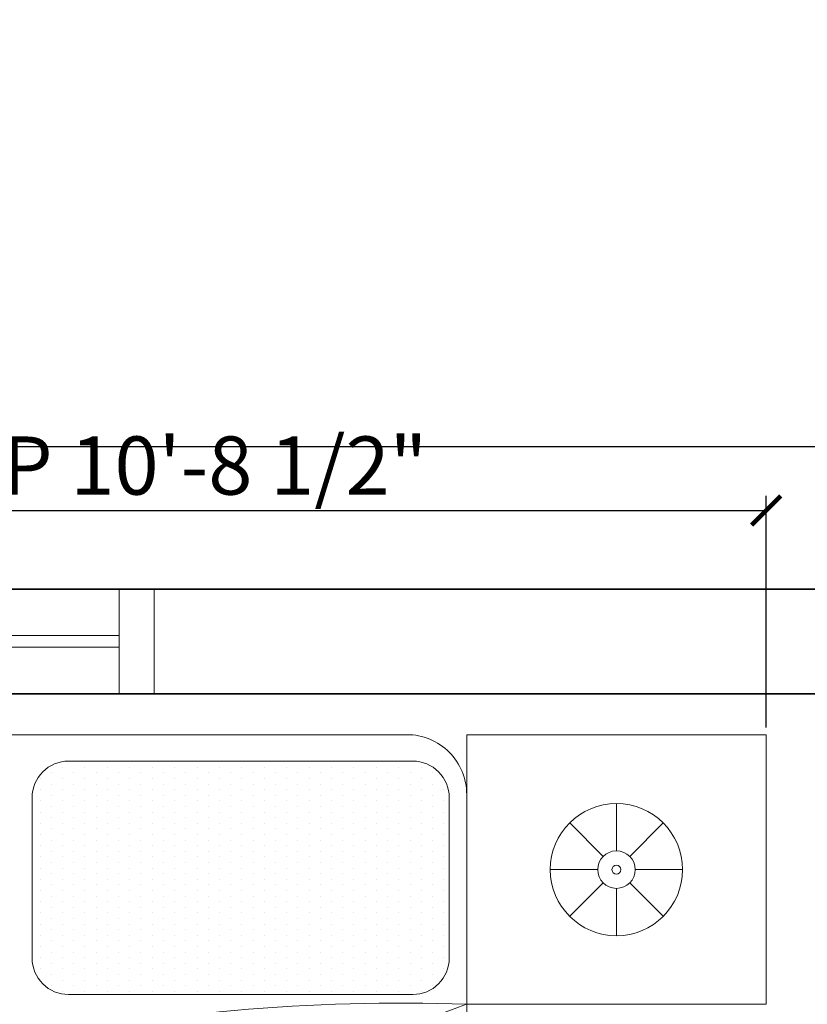
# Model space of a CAD drawing. Units: inches. Extents: x 3283068 to 3284536, y 3240756 to 3241803.
# Tile 11 of 19: x 3283453 to 3283520, y 3241603 to 3241688. Entities that reach past the tile are written whole.
import ezdxf

# ---------------------------------------------------------------- set-up
doc = ezdxf.new("R2010")
doc.units = ezdxf.units.IN
for name, color, linetype, lineweight in [('A-ANNO-DIMS', 2, 'Continuous', 18), ('furniture', 40, 'Continuous', 18), ('wall', 20, 'Continuous', 35), ('window', 100, 'Continuous', 18)]:
    doc.layers.add(name, color=color, linetype=linetype, lineweight=lineweight)
doc.styles.get("Standard").update_dxf_attribs({"font": 'arial.ttf'})
doc.dimstyles.new('ISO-25', dxfattribs={"dimtxt": 5, "dimasz": 2.5, "dimexe": 1.25, "dimexo": 0.625, "dimtad": 1, "dimlunit": 4, "dimtxsty": 'Standard', "dimblk": 'ARCHTICK', "dimcen": 2.5, "dimadec": 0, "dimazin": 0, "dimtfac": 1, "dimtmove": 0, "dimatfit": 3, "dimfxl": 1, "dimarcsym": 0})

# ---------------------------------------------------------------- blocks, each defined once
blk = doc.blocks.new('*X12')
at = {"color": 0}
for p, q in [((273.75, 456.9375), (273.75, 456.9375)), ((273.9375, 457.03125), (273.9375, 457.03125)), ((274.125, 456.9375), (274.125, 456.9375)), ((274.3125, 457.03125), (274.3125, 457.03125)), ((274.5, 456.9375), (274.5, 456.9375)), ((274.6875, 457.03125), (274.6875, 457.03125)), ((274.875, 456.9375), (274.875, 456.9375)), ((275.0625, 457.03125), (275.0625, 457.03125)), ((275.25, 456.9375), (275.25, 456.9375)), ((275.4375, 457.03125), (275.4375, 457.03125)), ((275.625, 456.9375), (275.625, 456.9375)), ((275.8125, 457.03125), (275.8125, 457.03125)), ((276, 456.9375), (276, 456.9375)), ((276.1875, 457.03125), (276.1875, 457.03125)), ((276.375, 456.9375), (276.375, 456.9375)), ((276.5625, 457.03125), (276.5625, 457.03125)), ((276.75, 456.9375), (276.75, 456.9375)), ((276.9375, 457.03125), (276.9375, 457.03125)), ((277.125, 456.9375), (277.125, 456.9375)), ((277.3125, 457.03125), (277.3125, 457.03125)), ((277.5, 456.9375), (277.5, 456.9375)), ((277.6875, 457.03125), (277.6875, 457.03125)), ((277.875, 456.9375), (277.875, 456.9375)), ((278.0625, 457.03125), (278.0625, 457.03125)), ((278.25, 456.9375), (278.25, 456.9375)), ((278.4375, 457.03125), (278.4375, 457.03125)), ((278.625, 456.9375), (278.625, 456.9375)), ((278.8125, 457.03125), (278.8125, 457.03125)), ((279, 456.9375), (279, 456.9375)), ((279.1875, 457.03125), (279.1875, 457.03125)), ((279.375, 456.9375), (279.375, 456.9375)), ((279.5625, 457.03125), (279.5625, 457.03125)), ((279.75, 456.9375), (279.75, 456.9375)), ((273.375, 456.75), (273.375, 456.75)), ((273.5625, 456.84375), (273.5625, 456.84375)), ((273.75, 456.75), (273.75, 456.75)), ((273.9375, 456.84375), (273.9375, 456.84375)), ((274.125, 456.75), (274.125, 456.75)), ((274.3125, 456.84375), (274.3125, 456.84375)), ((274.5, 456.75), (274.5, 456.75)), ((274.6875, 456.84375), (274.6875, 456.84375)), ((274.875, 456.75), (274.875, 456.75)), ((275.0625, 456.84375), (275.0625, 456.84375)), ((275.25, 456.75), (275.25, 456.75)), ((275.4375, 456.84375), (275.4375, 456.84375)), ((275.625, 456.75), (275.625, 456.75)), ((275.8125, 456.84375), (275.8125, 456.84375)), ((276, 456.75), (276, 456.75)), ((276.1875, 456.84375), (276.1875, 456.84375)), ((276.375, 456.75), (276.375, 456.75)), ((276.5625, 456.84375), (276.5625, 456.84375)), ((276.75, 456.75), (276.75, 456.75)), ((276.9375, 456.84375), (276.9375, 456.84375)), ((277.125, 456.75), (277.125, 456.75)), ((277.3125, 456.84375), (277.3125, 456.84375)), ((277.5, 456.75), (277.5, 456.75)), ((277.6875, 456.84375), (277.6875, 456.84375)), ((277.875, 456.75), (277.875, 456.75)), ((278.0625, 456.84375), (278.0625, 456.84375)), ((278.25, 456.75), (278.25, 456.75)), ((278.4375, 456.84375), (278.4375, 456.84375)), ((278.625, 456.75), (278.625, 456.75)), ((278.8125, 456.84375), (278.8125, 456.84375)), ((279, 456.75), (279, 456.75)), ((279.1875, 456.84375), (279.1875, 456.84375)), ((279.375, 456.75), (279.375, 456.75)), ((279.5625, 456.84375), (279.5625, 456.84375)), ((279.75, 456.75), (279.75, 456.75)), ((279.9375, 456.84375), (279.9375, 456.84375)), ((280.125, 456.75), (280.125, 456.75)), ((273.5625, 456.65625), (273.5625, 456.65625)), ((273.9375, 456.65625), (273.9375, 456.65625)), ((274.3125, 456.65625), (274.3125, 456.65625)), ((274.6875, 456.65625), (274.6875, 456.65625)), ((275.0625, 456.65625), (275.0625, 456.65625)), ((275.4375, 456.65625), (275.4375, 456.65625)), ((275.8125, 456.65625), (275.8125, 456.65625)), ((276.1875, 456.65625), (276.1875, 456.65625)), ((276.5625, 456.65625), (276.5625, 456.65625)), ((276.9375, 456.65625), (276.9375, 456.65625)), ((277.3125, 456.65625), (277.3125, 456.65625)), ((277.6875, 456.65625), (277.6875, 456.65625)), ((278.0625, 456.65625), (278.0625, 456.65625)), ((278.4375, 456.65625), (278.4375, 456.65625)), ((278.8125, 456.65625), (278.8125, 456.65625)), ((279.1875, 456.65625), (279.1875, 456.65625)), ((279.5625, 456.65625), (279.5625, 456.65625)), ((279.9375, 456.65625), (279.9375, 456.65625)), ((273.375, 456.5625), (273.375, 456.5625)), ((273.5625, 456.46875), (273.5625, 456.46875)), ((273.75, 456.5625), (273.75, 456.5625)), ((273.9375, 456.46875), (273.9375, 456.46875)), ((274.125, 456.5625), (274.125, 456.5625)), ((274.3125, 456.46875), (274.3125, 456.46875)), ((274.5, 456.5625), (274.5, 456.5625)), ((274.6875, 456.46875), (274.6875, 456.46875)), ((274.875, 456.5625), (274.875, 456.5625)), ((275.0625, 456.46875), (275.0625, 456.46875)), ((275.25, 456.5625), (275.25, 456.5625)), ((275.4375, 456.46875), (275.4375, 456.46875)), ((275.625, 456.5625), (275.625, 456.5625)), ((275.8125, 456.46875), (275.8125, 456.46875)), ((276, 456.5625), (276, 456.5625)), ((276.1875, 456.46875), (276.1875, 456.46875)), ((276.375, 456.5625), (276.375, 456.5625)), ((276.5625, 456.46875), (276.5625, 456.46875)), ((276.75, 456.5625), (276.75, 456.5625)), ((276.9375, 456.46875), (276.9375, 456.46875)), ((277.125, 456.5625), (277.125, 456.5625)), ((277.3125, 456.46875), (277.3125, 456.46875)), ((277.5, 456.5625), (277.5, 456.5625)), ((277.6875, 456.46875), (277.6875, 456.46875)), ((277.875, 456.5625), (277.875, 456.5625)), ((278.0625, 456.46875), (278.0625, 456.46875)), ((278.25, 456.5625), (278.25, 456.5625)), ((278.4375, 456.46875), (278.4375, 456.46875)), ((278.625, 456.5625), (278.625, 456.5625)), ((278.8125, 456.46875), (278.8125, 456.46875)), ((279, 456.5625), (279, 456.5625)), ((279.1875, 456.46875), (279.1875, 456.46875)), ((279.375, 456.5625), (279.375, 456.5625)), ((279.5625, 456.46875), (279.5625, 456.46875)), ((279.75, 456.5625), (279.75, 456.5625)), ((279.9375, 456.46875), (279.9375, 456.46875)), ((280.125, 456.5625), (280.125, 456.5625)), ((273.375, 456.375), (273.375, 456.375)), ((273.5625, 456.28125), (273.5625, 456.28125)), ((273.75, 456.375), (273.75, 456.375)), ((273.9375, 456.28125), (273.9375, 456.28125)), ((274.125, 456.375), (274.125, 456.375)), ((274.3125, 456.28125), (274.3125, 456.28125)), ((274.5, 456.375), (274.5, 456.375)), ((274.6875, 456.28125), (274.6875, 456.28125)), ((274.875, 456.375), (274.875, 456.375)), ((275.0625, 456.28125), (275.0625, 456.28125)), ((275.25, 456.375), (275.25, 456.375)), ((275.4375, 456.28125), (275.4375, 456.28125)), ((275.625, 456.375), (275.625, 456.375)), ((275.8125, 456.28125), (275.8125, 456.28125)), ((276, 456.375), (276, 456.375)), ((276.1875, 456.28125), (276.1875, 456.28125)), ((276.375, 456.375), (276.375, 456.375)), ((276.5625, 456.28125), (276.5625, 456.28125)), ((276.75, 456.375), (276.75, 456.375)), ((276.9375, 456.28125), (276.9375, 456.28125)), ((277.125, 456.375), (277.125, 456.375)), ((277.3125, 456.28125), (277.3125, 456.28125)), ((277.5, 456.375), (277.5, 456.375)), ((277.6875, 456.28125), (277.6875, 456.28125)), ((277.875, 456.375), (277.875, 456.375)), ((278.0625, 456.28125), (278.0625, 456.28125)), ((278.25, 456.375), (278.25, 456.375)), ((278.4375, 456.28125), (278.4375, 456.28125)), ((278.625, 456.375), (278.625, 456.375)), ((278.8125, 456.28125), (278.8125, 456.28125)), ((279, 456.375), (279, 456.375)), ((279.1875, 456.28125), (279.1875, 456.28125)), ((279.375, 456.375), (279.375, 456.375)), ((279.5625, 456.28125), (279.5625, 456.28125)), ((279.75, 456.375), (279.75, 456.375)), ((279.9375, 456.28125), (279.9375, 456.28125)), ((280.125, 456.375), (280.125, 456.375)), ((273.375, 456.1875), (273.375, 456.1875)), ((273.5625, 456.09375), (273.5625, 456.09375)), ((273.75, 456.1875), (273.75, 456.1875)), ((273.9375, 456.09375), (273.9375, 456.09375)), ((274.125, 456.1875), (274.125, 456.1875)), ((274.3125, 456.09375), (274.3125, 456.09375)), ((274.5, 456.1875), (274.5, 456.1875)), ((274.6875, 456.09375), (274.6875, 456.09375)), ((274.875, 456.1875), (274.875, 456.1875)), ((275.0625, 456.09375), (275.0625, 456.09375)), ((275.25, 456.1875), (275.25, 456.1875)), ((275.4375, 456.09375), (275.4375, 456.09375)), ((275.625, 456.1875), (275.625, 456.1875)), ((275.8125, 456.09375), (275.8125, 456.09375)), ((276, 456.1875), (276, 456.1875)), ((276.1875, 456.09375), (276.1875, 456.09375)), ((276.375, 456.1875), (276.375, 456.1875)), ((276.5625, 456.09375), (276.5625, 456.09375)), ((276.75, 456.1875), (276.75, 456.1875)), ((276.9375, 456.09375), (276.9375, 456.09375)), ((277.125, 456.1875), (277.125, 456.1875)), ((277.3125, 456.09375), (277.3125, 456.09375)), ((277.5, 456.1875), (277.5, 456.1875)), ((277.6875, 456.09375), (277.6875, 456.09375)), ((277.875, 456.1875), (277.875, 456.1875)), ((278.0625, 456.09375), (278.0625, 456.09375)), ((278.25, 456.1875), (278.25, 456.1875)), ((278.4375, 456.09375), (278.4375, 456.09375)), ((278.625, 456.1875), (278.625, 456.1875)), ((278.8125, 456.09375), (278.8125, 456.09375)), ((279, 456.1875), (279, 456.1875)), ((279.1875, 456.09375), (279.1875, 456.09375)), ((279.375, 456.1875), (279.375, 456.1875)), ((279.5625, 456.09375), (279.5625, 456.09375)), ((279.75, 456.1875), (279.75, 456.1875)), ((279.9375, 456.09375), (279.9375, 456.09375)), ((280.125, 456.1875), (280.125, 456.1875)), ((273.375, 456), (273.375, 456)), ((273.75, 456), (273.75, 456)), ((274.125, 456), (274.125, 456)), ((274.5, 456), (274.5, 456)), ((274.875, 456), (274.875, 456)), ((275.25, 456), (275.25, 456)), ((275.625, 456), (275.625, 456)), ((276, 456), (276, 456)), ((276.375, 456), (276.375, 456)), ((276.75, 456), (276.75, 456)), ((277.125, 456), (277.125, 456)), ((277.5, 456), (277.5, 456)), ((277.875, 456), (277.875, 456)), ((278.25, 456), (278.25, 456)), ((278.625, 456), (278.625, 456)), ((279, 456), (279, 456)), ((279.375, 456), (279.375, 456)), ((279.75, 456), (279.75, 456)), ((280.125, 456), (280.125, 456)), ((273.375, 455.8125), (273.375, 455.8125)), ((273.5625, 455.90625), (273.5625, 455.90625)), ((273.75, 455.8125), (273.75, 455.8125)), ((273.9375, 455.90625), (273.9375, 455.90625)), ((274.125, 455.8125), (274.125, 455.8125)), ((274.3125, 455.90625), (274.3125, 455.90625)), ((274.5, 455.8125), (274.5, 455.8125)), ((274.6875, 455.90625), (274.6875, 455.90625)), ((274.875, 455.8125), (274.875, 455.8125)), ((275.0625, 455.90625), (275.0625, 455.90625)), ((275.25, 455.8125), (275.25, 455.8125)), ((275.4375, 455.90625), (275.4375, 455.90625)), ((275.625, 455.8125), (275.625, 455.8125)), ((275.8125, 455.90625), (275.8125, 455.90625)), ((276, 455.8125), (276, 455.8125)), ((276.1875, 455.90625), (276.1875, 455.90625)), ((276.375, 455.8125), (276.375, 455.8125)), ((276.5625, 455.90625), (276.5625, 455.90625)), ((276.75, 455.8125), (276.75, 455.8125)), ((276.9375, 455.90625), (276.9375, 455.90625)), ((277.125, 455.8125), (277.125, 455.8125)), ((277.3125, 455.90625), (277.3125, 455.90625)), ((277.5, 455.8125), (277.5, 455.8125)), ((277.6875, 455.90625), (277.6875, 455.90625)), ((277.875, 455.8125), (277.875, 455.8125)), ((278.0625, 455.90625), (278.0625, 455.90625)), ((278.25, 455.8125), (278.25, 455.8125)), ((278.4375, 455.90625), (278.4375, 455.90625)), ((278.625, 455.8125), (278.625, 455.8125)), ((278.8125, 455.90625), (278.8125, 455.90625)), ((279, 455.8125), (279, 455.8125)), ((279.1875, 455.90625), (279.1875, 455.90625)), ((279.375, 455.8125), (279.375, 455.8125)), ((279.5625, 455.90625), (279.5625, 455.90625)), ((279.75, 455.8125), (279.75, 455.8125)), ((279.9375, 455.90625), (279.9375, 455.90625)), ((280.125, 455.8125), (280.125, 455.8125)), ((273.375, 455.625), (273.375, 455.625)), ((273.5625, 455.71875), (273.5625, 455.71875)), ((273.75, 455.625), (273.75, 455.625)), ((273.9375, 455.71875), (273.9375, 455.71875)), ((274.125, 455.625), (274.125, 455.625)), ((274.3125, 455.71875), (274.3125, 455.71875)), ((274.5, 455.625), (274.5, 455.625)), ((274.6875, 455.71875), (274.6875, 455.71875)), ((274.875, 455.625), (274.875, 455.625)), ((275.0625, 455.71875), (275.0625, 455.71875)), ((275.25, 455.625), (275.25, 455.625)), ((275.4375, 455.71875), (275.4375, 455.71875)), ((275.625, 455.625), (275.625, 455.625)), ((275.8125, 455.71875), (275.8125, 455.71875)), ((276, 455.625), (276, 455.625)), ((276.1875, 455.71875), (276.1875, 455.71875)), ((276.375, 455.625), (276.375, 455.625)), ((276.5625, 455.71875), (276.5625, 455.71875)), ((276.75, 455.625), (276.75, 455.625)), ((276.9375, 455.71875), (276.9375, 455.71875)), ((277.125, 455.625), (277.125, 455.625)), ((277.3125, 455.71875), (277.3125, 455.71875)), ((277.5, 455.625), (277.5, 455.625)), ((277.6875, 455.71875), (277.6875, 455.71875)), ((277.875, 455.625), (277.875, 455.625)), ((278.0625, 455.71875), (278.0625, 455.71875)), ((278.25, 455.625), (278.25, 455.625)), ((278.4375, 455.71875), (278.4375, 455.71875)), ((278.625, 455.625), (278.625, 455.625)), ((278.8125, 455.71875), (278.8125, 455.71875)), ((279, 455.625), (279, 455.625)), ((279.1875, 455.71875), (279.1875, 455.71875)), ((279.375, 455.625), (279.375, 455.625)), ((279.5625, 455.71875), (279.5625, 455.71875)), ((279.75, 455.625), (279.75, 455.625)), ((279.9375, 455.71875), (279.9375, 455.71875)), ((280.125, 455.625), (280.125, 455.625)), ((273.375, 455.4375), (273.375, 455.4375)), ((273.5625, 455.53125), (273.5625, 455.53125)), ((273.75, 455.4375), (273.75, 455.4375)), ((273.9375, 455.53125), (273.9375, 455.53125)), ((274.125, 455.4375), (274.125, 455.4375)), ((274.3125, 455.53125), (274.3125, 455.53125)), ((274.5, 455.4375), (274.5, 455.4375)), ((274.6875, 455.53125), (274.6875, 455.53125)), ((274.875, 455.4375), (274.875, 455.4375)), ((275.0625, 455.53125), (275.0625, 455.53125)), ((275.25, 455.4375), (275.25, 455.4375)), ((275.4375, 455.53125), (275.4375, 455.53125)), ((275.625, 455.4375), (275.625, 455.4375)), ((275.8125, 455.53125), (275.8125, 455.53125)), ((276, 455.4375), (276, 455.4375)), ((276.1875, 455.53125), (276.1875, 455.53125)), ((276.375, 455.4375), (276.375, 455.4375)), ((276.5625, 455.53125), (276.5625, 455.53125)), ((276.75, 455.4375), (276.75, 455.4375)), ((276.9375, 455.53125), (276.9375, 455.53125)), ((277.125, 455.4375), (277.125, 455.4375)), ((277.3125, 455.53125), (277.3125, 455.53125)), ((277.5, 455.4375), (277.5, 455.4375)), ((277.6875, 455.53125), (277.6875, 455.53125)), ((277.875, 455.4375), (277.875, 455.4375)), ((278.0625, 455.53125), (278.0625, 455.53125)), ((278.25, 455.4375), (278.25, 455.4375)), ((278.4375, 455.53125), (278.4375, 455.53125)), ((278.625, 455.4375), (278.625, 455.4375)), ((278.8125, 455.53125), (278.8125, 455.53125)), ((279, 455.4375), (279, 455.4375)), ((279.1875, 455.53125), (279.1875, 455.53125)), ((279.375, 455.4375), (279.375, 455.4375)), ((279.5625, 455.53125), (279.5625, 455.53125)), ((279.75, 455.4375), (279.75, 455.4375)), ((279.9375, 455.53125), (279.9375, 455.53125)), ((280.125, 455.4375), (280.125, 455.4375)), ((273.5625, 455.34375), (273.5625, 455.34375)), ((273.9375, 455.34375), (273.9375, 455.34375)), ((274.3125, 455.34375), (274.3125, 455.34375)), ((274.6875, 455.34375), (274.6875, 455.34375)), ((275.0625, 455.34375), (275.0625, 455.34375)), ((275.4375, 455.34375), (275.4375, 455.34375)), ((275.8125, 455.34375), (275.8125, 455.34375)), ((276.1875, 455.34375), (276.1875, 455.34375)), ((276.5625, 455.34375), (276.5625, 455.34375)), ((276.9375, 455.34375), (276.9375, 455.34375)), ((277.3125, 455.34375), (277.3125, 455.34375)), ((277.6875, 455.34375), (277.6875, 455.34375)), ((278.0625, 455.34375), (278.0625, 455.34375)), ((278.4375, 455.34375), (278.4375, 455.34375)), ((278.8125, 455.34375), (278.8125, 455.34375)), ((279.1875, 455.34375), (279.1875, 455.34375)), ((279.5625, 455.34375), (279.5625, 455.34375)), ((279.9375, 455.34375), (279.9375, 455.34375)), ((273.375, 455.25), (273.375, 455.25)), ((273.5625, 455.15625), (273.5625, 455.15625)), ((273.75, 455.25), (273.75, 455.25)), ((273.9375, 455.15625), (273.9375, 455.15625)), ((274.125, 455.25), (274.125, 455.25)), ((274.3125, 455.15625), (274.3125, 455.15625)), ((274.5, 455.25), (274.5, 455.25)), ((274.6875, 455.15625), (274.6875, 455.15625)), ((274.875, 455.25), (274.875, 455.25)), ((275.0625, 455.15625), (275.0625, 455.15625)), ((275.25, 455.25), (275.25, 455.25)), ((275.4375, 455.15625), (275.4375, 455.15625)), ((275.625, 455.25), (275.625, 455.25)), ((275.8125, 455.15625), (275.8125, 455.15625)), ((276, 455.25), (276, 455.25)), ((276.1875, 455.15625), (276.1875, 455.15625)), ((276.375, 455.25), (276.375, 455.25)), ((276.5625, 455.15625), (276.5625, 455.15625)), ((276.75, 455.25), (276.75, 455.25)), ((276.9375, 455.15625), (276.9375, 455.15625)), ((277.125, 455.25), (277.125, 455.25)), ((277.3125, 455.15625), (277.3125, 455.15625)), ((277.5, 455.25), (277.5, 455.25)), ((277.6875, 455.15625), (277.6875, 455.15625)), ((277.875, 455.25), (277.875, 455.25)), ((278.0625, 455.15625), (278.0625, 455.15625)), ((278.25, 455.25), (278.25, 455.25)), ((278.4375, 455.15625), (278.4375, 455.15625)), ((278.625, 455.25), (278.625, 455.25)), ((278.8125, 455.15625), (278.8125, 455.15625)), ((279, 455.25), (279, 455.25)), ((279.1875, 455.15625), (279.1875, 455.15625)), ((279.375, 455.25), (279.375, 455.25)), ((279.5625, 455.15625), (279.5625, 455.15625)), ((279.75, 455.25), (279.75, 455.25)), ((279.9375, 455.15625), (279.9375, 455.15625)), ((280.125, 455.25), (280.125, 455.25)), ((273.375, 455.0625), (273.375, 455.0625)), ((273.5625, 454.96875), (273.5625, 454.96875)), ((273.75, 455.0625), (273.75, 455.0625)), ((273.9375, 454.96875), (273.9375, 454.96875)), ((274.125, 455.0625), (274.125, 455.0625)), ((274.3125, 454.96875), (274.3125, 454.96875)), ((274.5, 455.0625), (274.5, 455.0625)), ((274.6875, 454.96875), (274.6875, 454.96875)), ((274.875, 455.0625), (274.875, 455.0625)), ((275.0625, 454.96875), (275.0625, 454.96875)), ((275.25, 455.0625), (275.25, 455.0625)), ((275.4375, 454.96875), (275.4375, 454.96875)), ((275.625, 455.0625), (275.625, 455.0625)), ((275.8125, 454.96875), (275.8125, 454.96875)), ((276, 455.0625), (276, 455.0625)), ((276.1875, 454.96875), (276.1875, 454.96875)), ((276.375, 455.0625), (276.375, 455.0625)), ((276.5625, 454.96875), (276.5625, 454.96875)), ((276.75, 455.0625), (276.75, 455.0625)), ((276.9375, 454.96875), (276.9375, 454.96875)), ((277.125, 455.0625), (277.125, 455.0625)), ((277.3125, 454.96875), (277.3125, 454.96875)), ((277.5, 455.0625), (277.5, 455.0625)), ((277.6875, 454.96875), (277.6875, 454.96875)), ((277.875, 455.0625), (277.875, 455.0625)), ((278.0625, 454.96875), (278.0625, 454.96875)), ((278.25, 455.0625), (278.25, 455.0625)), ((278.4375, 454.96875), (278.4375, 454.96875)), ((278.625, 455.0625), (278.625, 455.0625)), ((278.8125, 454.96875), (278.8125, 454.96875)), ((279, 455.0625), (279, 455.0625)), ((279.1875, 454.96875), (279.1875, 454.96875)), ((279.375, 455.0625), (279.375, 455.0625)), ((279.5625, 454.96875), (279.5625, 454.96875)), ((279.75, 455.0625), (279.75, 455.0625)), ((279.9375, 454.96875), (279.9375, 454.96875)), ((280.125, 455.0625), (280.125, 455.0625)), ((273.375, 454.875), (273.375, 454.875)), ((273.5625, 454.78125), (273.5625, 454.78125)), ((273.75, 454.875), (273.75, 454.875)), ((273.9375, 454.78125), (273.9375, 454.78125)), ((274.125, 454.875), (274.125, 454.875)), ((274.3125, 454.78125), (274.3125, 454.78125)), ((274.5, 454.875), (274.5, 454.875)), ((274.6875, 454.78125), (274.6875, 454.78125)), ((274.875, 454.875), (274.875, 454.875)), ((275.0625, 454.78125), (275.0625, 454.78125)), ((275.25, 454.875), (275.25, 454.875)), ((275.4375, 454.78125), (275.4375, 454.78125)), ((275.625, 454.875), (275.625, 454.875)), ((275.8125, 454.78125), (275.8125, 454.78125)), ((276, 454.875), (276, 454.875)), ((276.1875, 454.78125), (276.1875, 454.78125)), ((276.375, 454.875), (276.375, 454.875)), ((276.5625, 454.78125), (276.5625, 454.78125)), ((276.75, 454.875), (276.75, 454.875)), ((276.9375, 454.78125), (276.9375, 454.78125)), ((277.125, 454.875), (277.125, 454.875)), ((277.3125, 454.78125), (277.3125, 454.78125)), ((277.5, 454.875), (277.5, 454.875)), ((277.6875, 454.78125), (277.6875, 454.78125)), ((277.875, 454.875), (277.875, 454.875)), ((278.0625, 454.78125), (278.0625, 454.78125)), ((278.25, 454.875), (278.25, 454.875)), ((278.4375, 454.78125), (278.4375, 454.78125)), ((278.625, 454.875), (278.625, 454.875)), ((278.8125, 454.78125), (278.8125, 454.78125)), ((279, 454.875), (279, 454.875)), ((279.1875, 454.78125), (279.1875, 454.78125)), ((279.375, 454.875), (279.375, 454.875)), ((279.5625, 454.78125), (279.5625, 454.78125)), ((279.75, 454.875), (279.75, 454.875)), ((279.9375, 454.78125), (279.9375, 454.78125)), ((280.125, 454.875), (280.125, 454.875)), ((273.375, 454.6875), (273.375, 454.6875)), ((273.75, 454.6875), (273.75, 454.6875)), ((274.125, 454.6875), (274.125, 454.6875)), ((274.5, 454.6875), (274.5, 454.6875)), ((274.875, 454.6875), (274.875, 454.6875)), ((275.25, 454.6875), (275.25, 454.6875)), ((275.625, 454.6875), (275.625, 454.6875)), ((276, 454.6875), (276, 454.6875)), ((276.375, 454.6875), (276.375, 454.6875)), ((276.75, 454.6875), (276.75, 454.6875)), ((277.125, 454.6875), (277.125, 454.6875)), ((277.5, 454.6875), (277.5, 454.6875)), ((277.875, 454.6875), (277.875, 454.6875)), ((278.25, 454.6875), (278.25, 454.6875)), ((278.625, 454.6875), (278.625, 454.6875)), ((279, 454.6875), (279, 454.6875)), ((279.375, 454.6875), (279.375, 454.6875)), ((279.75, 454.6875), (279.75, 454.6875)), ((280.125, 454.6875), (280.125, 454.6875)), ((273.375, 454.5), (273.375, 454.5)), ((273.5625, 454.59375), (273.5625, 454.59375)), ((273.75, 454.5), (273.75, 454.5)), ((273.9375, 454.59375), (273.9375, 454.59375)), ((274.125, 454.5), (274.125, 454.5)), ((274.3125, 454.59375), (274.3125, 454.59375)), ((274.5, 454.5), (274.5, 454.5)), ((274.6875, 454.59375), (274.6875, 454.59375)), ((274.875, 454.5), (274.875, 454.5)), ((275.0625, 454.59375), (275.0625, 454.59375)), ((275.25, 454.5), (275.25, 454.5)), ((275.4375, 454.59375), (275.4375, 454.59375)), ((275.625, 454.5), (275.625, 454.5)), ((275.8125, 454.59375), (275.8125, 454.59375)), ((276, 454.5), (276, 454.5)), ((276.1875, 454.59375), (276.1875, 454.59375)), ((276.375, 454.5), (276.375, 454.5)), ((276.5625, 454.59375), (276.5625, 454.59375)), ((276.75, 454.5), (276.75, 454.5)), ((276.9375, 454.59375), (276.9375, 454.59375)), ((277.125, 454.5), (277.125, 454.5)), ((277.3125, 454.59375), (277.3125, 454.59375)), ((277.5, 454.5), (277.5, 454.5)), ((277.6875, 454.59375), (277.6875, 454.59375)), ((277.875, 454.5), (277.875, 454.5)), ((278.0625, 454.59375), (278.0625, 454.59375)), ((278.25, 454.5), (278.25, 454.5)), ((278.4375, 454.59375), (278.4375, 454.59375)), ((278.625, 454.5), (278.625, 454.5)), ((278.8125, 454.59375), (278.8125, 454.59375)), ((279, 454.5), (279, 454.5)), ((279.1875, 454.59375), (279.1875, 454.59375)), ((279.375, 454.5), (279.375, 454.5)), ((279.5625, 454.59375), (279.5625, 454.59375)), ((279.75, 454.5), (279.75, 454.5)), ((279.9375, 454.59375), (279.9375, 454.59375)), ((280.125, 454.5), (280.125, 454.5)), ((273.375, 454.3125), (273.375, 454.3125)), ((273.5625, 454.40625), (273.5625, 454.40625)), ((273.75, 454.3125), (273.75, 454.3125)), ((273.9375, 454.40625), (273.9375, 454.40625)), ((274.125, 454.3125), (274.125, 454.3125)), ((274.3125, 454.40625), (274.3125, 454.40625)), ((274.5, 454.3125), (274.5, 454.3125)), ((274.6875, 454.40625), (274.6875, 454.40625)), ((274.875, 454.3125), (274.875, 454.3125)), ((275.0625, 454.40625), (275.0625, 454.40625)), ((275.25, 454.3125), (275.25, 454.3125)), ((275.4375, 454.40625), (275.4375, 454.40625)), ((275.625, 454.3125), (275.625, 454.3125)), ((275.8125, 454.40625), (275.8125, 454.40625)), ((276, 454.3125), (276, 454.3125)), ((276.1875, 454.40625), (276.1875, 454.40625)), ((276.375, 454.3125), (276.375, 454.3125)), ((276.5625, 454.40625), (276.5625, 454.40625)), ((276.75, 454.3125), (276.75, 454.3125)), ((276.9375, 454.40625), (276.9375, 454.40625)), ((277.125, 454.3125), (277.125, 454.3125)), ((277.3125, 454.40625), (277.3125, 454.40625)), ((277.5, 454.3125), (277.5, 454.3125)), ((277.6875, 454.40625), (277.6875, 454.40625)), ((277.875, 454.3125), (277.875, 454.3125)), ((278.0625, 454.40625), (278.0625, 454.40625)), ((278.25, 454.3125), (278.25, 454.3125)), ((278.4375, 454.40625), (278.4375, 454.40625)), ((278.625, 454.3125), (278.625, 454.3125)), ((278.8125, 454.40625), (278.8125, 454.40625)), ((279, 454.3125), (279, 454.3125)), ((279.1875, 454.40625), (279.1875, 454.40625)), ((279.375, 454.3125), (279.375, 454.3125)), ((279.5625, 454.40625), (279.5625, 454.40625)), ((279.75, 454.3125), (279.75, 454.3125)), ((279.9375, 454.40625), (279.9375, 454.40625)), ((280.125, 454.3125), (280.125, 454.3125)), ((273.375, 454.125), (273.375, 454.125)), ((273.5625, 454.21875), (273.5625, 454.21875)), ((273.75, 454.125), (273.75, 454.125)), ((273.9375, 454.21875), (273.9375, 454.21875)), ((274.125, 454.125), (274.125, 454.125)), ((274.3125, 454.21875), (274.3125, 454.21875)), ((274.5, 454.125), (274.5, 454.125)), ((274.6875, 454.21875), (274.6875, 454.21875)), ((274.875, 454.125), (274.875, 454.125)), ((275.0625, 454.21875), (275.0625, 454.21875)), ((275.25, 454.125), (275.25, 454.125)), ((275.4375, 454.21875), (275.4375, 454.21875)), ((275.625, 454.125), (275.625, 454.125)), ((275.8125, 454.21875), (275.8125, 454.21875)), ((276, 454.125), (276, 454.125)), ((276.1875, 454.21875), (276.1875, 454.21875)), ((276.375, 454.125), (276.375, 454.125)), ((276.5625, 454.21875), (276.5625, 454.21875)), ((276.75, 454.125), (276.75, 454.125)), ((276.9375, 454.21875), (276.9375, 454.21875)), ((277.125, 454.125), (277.125, 454.125)), ((277.3125, 454.21875), (277.3125, 454.21875)), ((277.5, 454.125), (277.5, 454.125)), ((277.6875, 454.21875), (277.6875, 454.21875)), ((277.875, 454.125), (277.875, 454.125)), ((278.0625, 454.21875), (278.0625, 454.21875)), ((278.25, 454.125), (278.25, 454.125)), ((278.4375, 454.21875), (278.4375, 454.21875)), ((278.625, 454.125), (278.625, 454.125)), ((278.8125, 454.21875), (278.8125, 454.21875)), ((279, 454.125), (279, 454.125)), ((279.1875, 454.21875), (279.1875, 454.21875)), ((279.375, 454.125), (279.375, 454.125)), ((279.5625, 454.21875), (279.5625, 454.21875)), ((279.75, 454.125), (279.75, 454.125)), ((279.9375, 454.21875), (279.9375, 454.21875)), ((280.125, 454.125), (280.125, 454.125)), ((273.5625, 454.03125), (273.5625, 454.03125)), ((273.9375, 454.03125), (273.9375, 454.03125)), ((274.3125, 454.03125), (274.3125, 454.03125)), ((274.6875, 454.03125), (274.6875, 454.03125)), ((275.0625, 454.03125), (275.0625, 454.03125)), ((275.4375, 454.03125), (275.4375, 454.03125)), ((275.8125, 454.03125), (275.8125, 454.03125)), ((276.1875, 454.03125), (276.1875, 454.03125)), ((276.5625, 454.03125), (276.5625, 454.03125)), ((276.9375, 454.03125), (276.9375, 454.03125)), ((277.3125, 454.03125), (277.3125, 454.03125)), ((277.6875, 454.03125), (277.6875, 454.03125)), ((278.0625, 454.03125), (278.0625, 454.03125)), ((278.4375, 454.03125), (278.4375, 454.03125)), ((278.8125, 454.03125), (278.8125, 454.03125)), ((279.1875, 454.03125), (279.1875, 454.03125)), ((279.5625, 454.03125), (279.5625, 454.03125)), ((279.9375, 454.03125), (279.9375, 454.03125)), ((273.375, 453.9375), (273.375, 453.9375)), ((273.5625, 453.84375), (273.5625, 453.84375)), ((273.75, 453.9375), (273.75, 453.9375)), ((273.9375, 453.84375), (273.9375, 453.84375)), ((274.125, 453.9375), (274.125, 453.9375)), ((274.3125, 453.84375), (274.3125, 453.84375)), ((274.5, 453.9375), (274.5, 453.9375)), ((274.6875, 453.84375), (274.6875, 453.84375)), ((274.875, 453.9375), (274.875, 453.9375)), ((275.0625, 453.84375), (275.0625, 453.84375)), ((275.25, 453.9375), (275.25, 453.9375)), ((275.4375, 453.84375), (275.4375, 453.84375)), ((275.625, 453.9375), (275.625, 453.9375)), ((275.8125, 453.84375), (275.8125, 453.84375)), ((276, 453.9375), (276, 453.9375)), ((276.1875, 453.84375), (276.1875, 453.84375)), ((276.375, 453.9375), (276.375, 453.9375)), ((276.5625, 453.84375), (276.5625, 453.84375)), ((276.75, 453.9375), (276.75, 453.9375)), ((276.9375, 453.84375), (276.9375, 453.84375)), ((277.125, 453.9375), (277.125, 453.9375)), ((277.3125, 453.84375), (277.3125, 453.84375)), ((277.5, 453.9375), (277.5, 453.9375)), ((277.6875, 453.84375), (277.6875, 453.84375)), ((277.875, 453.9375), (277.875, 453.9375)), ((278.0625, 453.84375), (278.0625, 453.84375)), ((278.25, 453.9375), (278.25, 453.9375)), ((278.4375, 453.84375), (278.4375, 453.84375)), ((278.625, 453.9375), (278.625, 453.9375)), ((278.8125, 453.84375), (278.8125, 453.84375)), ((279, 453.9375), (279, 453.9375)), ((279.1875, 453.84375), (279.1875, 453.84375)), ((279.375, 453.9375), (279.375, 453.9375)), ((279.5625, 453.84375), (279.5625, 453.84375)), ((279.75, 453.9375), (279.75, 453.9375)), ((279.9375, 453.84375), (279.9375, 453.84375)), ((280.125, 453.9375), (280.125, 453.9375)), ((273.375, 453.75), (273.375, 453.75)), ((273.5625, 453.65625), (273.5625, 453.65625)), ((273.75, 453.75), (273.75, 453.75)), ((273.9375, 453.65625), (273.9375, 453.65625)), ((274.125, 453.75), (274.125, 453.75)), ((274.3125, 453.65625), (274.3125, 453.65625)), ((274.5, 453.75), (274.5, 453.75)), ((274.6875, 453.65625), (274.6875, 453.65625)), ((274.875, 453.75), (274.875, 453.75)), ((275.0625, 453.65625), (275.0625, 453.65625)), ((275.25, 453.75), (275.25, 453.75)), ((275.4375, 453.65625), (275.4375, 453.65625)), ((275.625, 453.75), (275.625, 453.75)), ((275.8125, 453.65625), (275.8125, 453.65625)), ((276, 453.75), (276, 453.75)), ((276.1875, 453.65625), (276.1875, 453.65625)), ((276.375, 453.75), (276.375, 453.75)), ((276.5625, 453.65625), (276.5625, 453.65625)), ((276.75, 453.75), (276.75, 453.75)), ((276.9375, 453.65625), (276.9375, 453.65625)), ((277.125, 453.75), (277.125, 453.75)), ((277.3125, 453.65625), (277.3125, 453.65625)), ((277.5, 453.75), (277.5, 453.75)), ((277.6875, 453.65625), (277.6875, 453.65625)), ((277.875, 453.75), (277.875, 453.75)), ((278.0625, 453.65625), (278.0625, 453.65625)), ((278.25, 453.75), (278.25, 453.75)), ((278.4375, 453.65625), (278.4375, 453.65625)), ((278.625, 453.75), (278.625, 453.75)), ((278.8125, 453.65625), (278.8125, 453.65625)), ((279, 453.75), (279, 453.75)), ((279.1875, 453.65625), (279.1875, 453.65625)), ((279.375, 453.75), (279.375, 453.75)), ((279.5625, 453.65625), (279.5625, 453.65625)), ((279.75, 453.75), (279.75, 453.75)), ((279.9375, 453.65625), (279.9375, 453.65625)), ((280.125, 453.75), (280.125, 453.75)), ((273.375, 453.5625), (273.375, 453.5625)), ((273.5625, 453.46875), (273.5625, 453.46875)), ((273.75, 453.5625), (273.75, 453.5625)), ((273.9375, 453.46875), (273.9375, 453.46875)), ((274.125, 453.5625), (274.125, 453.5625)), ((274.3125, 453.46875), (274.3125, 453.46875)), ((274.5, 453.5625), (274.5, 453.5625)), ((274.6875, 453.46875), (274.6875, 453.46875)), ((274.875, 453.5625), (274.875, 453.5625)), ((275.0625, 453.46875), (275.0625, 453.46875)), ((275.25, 453.5625), (275.25, 453.5625)), ((275.4375, 453.46875), (275.4375, 453.46875)), ((275.625, 453.5625), (275.625, 453.5625)), ((275.8125, 453.46875), (275.8125, 453.46875)), ((276, 453.5625), (276, 453.5625)), ((276.1875, 453.46875), (276.1875, 453.46875)), ((276.375, 453.5625), (276.375, 453.5625)), ((276.5625, 453.46875), (276.5625, 453.46875)), ((276.75, 453.5625), (276.75, 453.5625)), ((276.9375, 453.46875), (276.9375, 453.46875)), ((277.125, 453.5625), (277.125, 453.5625)), ((277.3125, 453.46875), (277.3125, 453.46875)), ((277.5, 453.5625), (277.5, 453.5625)), ((277.6875, 453.46875), (277.6875, 453.46875)), ((277.875, 453.5625), (277.875, 453.5625)), ((278.0625, 453.46875), (278.0625, 453.46875)), ((278.25, 453.5625), (278.25, 453.5625)), ((278.4375, 453.46875), (278.4375, 453.46875)), ((278.625, 453.5625), (278.625, 453.5625)), ((278.8125, 453.46875), (278.8125, 453.46875)), ((279, 453.5625), (279, 453.5625)), ((279.1875, 453.46875), (279.1875, 453.46875)), ((279.375, 453.5625), (279.375, 453.5625)), ((279.5625, 453.46875), (279.5625, 453.46875)), ((279.75, 453.5625), (279.75, 453.5625)), ((279.9375, 453.46875), (279.9375, 453.46875)), ((280.125, 453.5625), (280.125, 453.5625)), ((273.375, 453.375), (273.375, 453.375)), ((273.75, 453.375), (273.75, 453.375)), ((274.125, 453.375), (274.125, 453.375)), ((274.5, 453.375), (274.5, 453.375)), ((274.875, 453.375), (274.875, 453.375)), ((275.25, 453.375), (275.25, 453.375)), ((275.625, 453.375), (275.625, 453.375)), ((276, 453.375), (276, 453.375)), ((276.375, 453.375), (276.375, 453.375)), ((276.75, 453.375), (276.75, 453.375)), ((277.125, 453.375), (277.125, 453.375)), ((277.5, 453.375), (277.5, 453.375)), ((277.875, 453.375), (277.875, 453.375)), ((278.25, 453.375), (278.25, 453.375)), ((278.625, 453.375), (278.625, 453.375)), ((279, 453.375), (279, 453.375)), ((279.375, 453.375), (279.375, 453.375)), ((279.75, 453.375), (279.75, 453.375)), ((273.5625, 453.28125), (273.5625, 453.28125)), ((273.75, 453.1875), (273.75, 453.1875)), ((273.9375, 453.28125), (273.9375, 453.28125)), ((274.125, 453.1875), (274.125, 453.1875)), ((274.3125, 453.28125), (274.3125, 453.28125)), ((274.5, 453.1875), (274.5, 453.1875)), ((274.6875, 453.28125), (274.6875, 453.28125)), ((274.875, 453.1875), (274.875, 453.1875)), ((275.0625, 453.28125), (275.0625, 453.28125)), ((275.25, 453.1875), (275.25, 453.1875)), ((275.4375, 453.28125), (275.4375, 453.28125)), ((275.625, 453.1875), (275.625, 453.1875)), ((275.8125, 453.28125), (275.8125, 453.28125)), ((276, 453.1875), (276, 453.1875)), ((276.1875, 453.28125), (276.1875, 453.28125)), ((276.375, 453.1875), (276.375, 453.1875)), ((276.5625, 453.28125), (276.5625, 453.28125)), ((276.75, 453.1875), (276.75, 453.1875)), ((276.9375, 453.28125), (276.9375, 453.28125)), ((277.125, 453.1875), (277.125, 453.1875)), ((277.3125, 453.28125), (277.3125, 453.28125)), ((277.5, 453.1875), (277.5, 453.1875)), ((277.6875, 453.28125), (277.6875, 453.28125)), ((277.875, 453.1875), (277.875, 453.1875)), ((278.0625, 453.28125), (278.0625, 453.28125)), ((278.25, 453.1875), (278.25, 453.1875)), ((278.4375, 453.28125), (278.4375, 453.28125)), ((278.625, 453.1875), (278.625, 453.1875)), ((278.8125, 453.28125), (278.8125, 453.28125)), ((279, 453.1875), (279, 453.1875)), ((279.1875, 453.28125), (279.1875, 453.28125)), ((279.375, 453.1875), (279.375, 453.1875)), ((279.5625, 453.28125), (279.5625, 453.28125)), ((279.75, 453.1875), (279.75, 453.1875)), ((279.9375, 453.28125), (279.9375, 453.28125))]:
    blk.add_line(p, q, dxfattribs=at)
blk = doc.blocks.new('A$C52E67D0D')
at = {"layer": 'furniture'}
for p, q in [((2251.5, 1605.5), (2251.5, 1684.7)), ((2229.3, 1596.3), (2173.3, 1652.3)), ((2273.7, 1596.3), (2329.7, 1652.3)), ((2220.1, 1574.1), (2140.9, 1574.1)), ((2282.9, 1574.1), (2362.1, 1574.1)), ((2229.3, 1551.9), (2173.3, 1495.9)), ((2273.7, 1551.9), (2329.7, 1495.9)), ((2251.5, 1542.8), (2251.5, 1463.5))]:
    blk.add_line(p, q, dxfattribs=at)
for points in [[(1901, 0), (601, 0, -0.414214), (501, 100), (501, 1700, -0.414214), (601, 1800), (1901, 1800, -0.414214), (2001, 1700), (2001, 100, -0.414214)], [(1911, 1365.1), (1335, 1365.1, -0.414214), (1274.2, 1425.9), (1274.2, 1694.8, -0.414214), (1335, 1755.7), (1911, 1755.7, -0.414214), (1971.8, 1694.8), (1971.8, 1425.9, -0.414214)]]:
    blk.add_lwpolyline(points, format="xyb", close=True, dxfattribs=at)
blk.add_lwpolyline([(2001, 1348.6), (2001, 1799.6), (2502, 1799.6), (2502, 1348.6)], close=True, dxfattribs=at)
for radius in [110.6, 31.4, 7.46]:
    blk.add_circle((2251.5, 1574.1), radius, dxfattribs=at)
for centre, radius, start, end in [((1888.6, -1664.5), 3015.3, 87.8642, 117.4001), ((3101, -1685.8), 3227.7, 109.926, 135.3977)]:
    blk.add_arc(centre, radius, start, end, dxfattribs=at)
at = {"layer": 'furniture', "xscale": 100, "yscale": 100, "zscale": 100}
blk.add_blockref('*X12', (-26050, -43948.2), dxfattribs=at)
blk = doc.blocks.new('_ArchTick')
at = {"color": 0, "linetype": 'ByBlock', "const_width": 0.15}
blk.add_lwpolyline([(-0.5, -0.5), (0.5, 0.5)], dxfattribs=at)
blk = doc.blocks.new('*D25')
at = {"layer": 'A-ANNO-DIMS', "color": 0, "lineweight": -2, "transparency": 16777216}
for p, q in [((3283339.589, 3241639.727), (3283339.589, 3241652.584)), ((3284236.589, 3241639.727), (3284236.589, 3241652.584)), ((3283339.589, 3241651.334), (3284236.589, 3241651.334))]:
    blk.add_line(p, q, dxfattribs=at)
at = {"layer": 'Defpoints', "color": 0, "transparency": 16777216}
for p in [(3284236.589, 3241651.334), (3283339.589, 3241639.102), (3284236.589, 3241639.102)]:
    blk.add_point(p, dxfattribs=at)
at = {"layer": 'A-ANNO-DIMS', "color": 0, "lineweight": -2, "transparency": 16777216, "xscale": 2.5, "yscale": 2.5, "zscale": 2.5, "rotation": 180}
blk.add_blockref('_ArchTick', (3283339.589, 3241651.334), dxfattribs=at)
at = {"layer": 'A-ANNO-DIMS', "color": 0, "lineweight": -2, "transparency": 16777216, "xscale": 2.5, "yscale": 2.5, "zscale": 2.5}
blk.add_blockref('_ArchTick', (3284236.589, 3241651.334), dxfattribs=at)
at = {"layer": 'A-ANNO-DIMS', "color": 0, "transparency": 16777216, "insert": (3283788.089, 3241654.512), "char_height": 5, "attachment_point": 5}
blk.add_mtext('74\'-9"', dxfattribs=at)
blk = doc.blocks.new('WIN-48IN-9IN-WALL')
for p, q in [((0, 9), (48, 9)), ((0, 0), (0, 9)), ((3, 0), (3, 9)), ((45, 9), (45, 0)), ((48, 9), (48, 0)), ((3, 5), (45, 5)), ((3, 4), (45, 4)), ((48, 0), (0, 0))]:
    blk.add_line(p, q)
blk = doc.blocks.new('*D57')
at = {"layer": 'A-ANNO-DIMS', "color": 0, "lineweight": -2, "transparency": 16777216}
for p, q in [((3283388.229, 3241627.215), (3283388.229, 3241647.098)), ((3283516.614, 3241627.215), (3283516.614, 3241647.098)), ((3283388.229, 3241645.848), (3283516.614, 3241645.848))]:
    blk.add_line(p, q, dxfattribs=at)
at = {"layer": 'Defpoints', "color": 0, "transparency": 16777216}
for p in [(3283516.614, 3241645.848), (3283388.229, 3241626.59), (3283516.614, 3241626.59)]:
    blk.add_point(p, dxfattribs=at)
at = {"layer": 'A-ANNO-DIMS', "color": 0, "lineweight": -2, "transparency": 16777216, "xscale": 2.5, "yscale": 2.5, "zscale": 2.5, "rotation": 180}
blk.add_blockref('_ArchTick', (3283388.229, 3241645.848), dxfattribs=at)
at = {"layer": 'A-ANNO-DIMS', "color": 0, "lineweight": -2, "transparency": 16777216, "xscale": 2.5, "yscale": 2.5, "zscale": 2.5}
blk.add_blockref('_ArchTick', (3283516.614, 3241645.848), dxfattribs=at)
at = {"layer": 'A-ANNO-DIMS', "color": 0, "transparency": 16777216, "insert": (3283452.421, 3241649.06), "char_height": 5, "attachment_point": 5}
blk.add_mtext('BED GROUP 10\'-8 1/2"', dxfattribs=at)
blk = doc.blocks.new('*D63')
at = {"layer": 'A-ANNO-DIMS', "color": 0, "lineweight": -2, "transparency": 16777216}
for p, q in [((3283248.089, 3241083.227), (3283248.089, 3241798.077)), ((3284328.089, 3241083.227), (3284328.089, 3241798.077)), ((3283248.089, 3241796.827), (3284328.089, 3241796.827))]:
    blk.add_line(p, q, dxfattribs=at)
at = {"layer": 'Defpoints', "color": 0, "transparency": 16777216}
for p in [(3284328.089, 3241796.827), (3283248.089, 3241082.602), (3284328.089, 3241082.602)]:
    blk.add_point(p, dxfattribs=at)
at = {"layer": 'A-ANNO-DIMS', "color": 0, "lineweight": -2, "transparency": 16777216, "xscale": 2.5, "yscale": 2.5, "zscale": 2.5, "rotation": 180}
blk.add_blockref('_ArchTick', (3283248.089, 3241796.827), dxfattribs=at)
at = {"layer": 'A-ANNO-DIMS', "color": 0, "lineweight": -2, "transparency": 16777216, "xscale": 2.5, "yscale": 2.5, "zscale": 2.5}
blk.add_blockref('_ArchTick', (3284328.089, 3241796.827), dxfattribs=at)
at = {"layer": 'A-ANNO-DIMS', "color": 0, "transparency": 16777216, "insert": (3283788.089, 3241800.005), "char_height": 5, "attachment_point": 5}
blk.add_mtext('90\'-0"', dxfattribs=at)

msp = doc.modelspace()

# ---------------------------------------------------------------- linework, layer by layer
at = {"layer": 'wall'}
for p, q in [((3283339.589, 3241639.102), (3284236.589, 3241639.102)), ((3283348.589, 3241630.102), (3283531.589, 3241630.102))]:
    msp.add_line(p, q, dxfattribs=at)

# ---------------------------------------------------------------- block references
at = {"layer": 'furniture', "xscale": 0.0513129658560468, "yscale": 0.0513129658560468, "zscale": 0.0513129658560468}
msp.add_blockref('A$C52E67D0D', (3283388.229, 3241534.227), dxfattribs=at)
at = {"layer": 'window'}
msp.add_blockref('WIN-48IN-9IN-WALL', (3283416.089, 3241630.102), dxfattribs=at)

# ---------------------------------------------------------------- dimensions: what is measured, and where the dimension line sits
at = {"layer": 'A-ANNO-DIMS'}
for base, p1, p2, override, picture, middle in [((3284328.089, 3241796.827), (3283248.089, 3241082.602), (3284328.089, 3241082.602), {"dimdec": 1, "dimlfac": 1, "dimrnd": 0, "dimzin": 1, "dimdsep": 46, "dimlunit": 4, "dimfrac": 2}, '*D63', (3283788.089, 3241800.005)), ((3284236.589, 3241651.334), (3283339.589, 3241639.102), (3284236.589, 3241639.102), {"dimclrd": 0, "dimclre": 0, "dimclrt": 0}, '*D25', (3283788.089, 3241654.512))]:
    dim = msp.add_linear_dim(base=base, p1=p1, p2=p2, dimstyle='ISO-25', override=override, dxfattribs=at)
    dim.commit()
    dim.dimension.update_dxf_attribs({"geometry": picture, "text_midpoint": middle})
dim = msp.add_linear_dim(base=(3283516.614, 3241645.848), p1=(3283388.229, 3241626.59), p2=(3283516.614, 3241626.59), text='BED GROUP <>', dimstyle='ISO-25', override={"dimdec": 1, "dimlfac": 1, "dimrnd": 0, "dimzin": 1, "dimdsep": 46, "dimlunit": 4, "dimfrac": 2}, dxfattribs=at)
dim.commit()
dim.dimension.update_dxf_attribs({"geometry": '*D57', "text_midpoint": (3283452.421, 3241649.06)})

doc.saveas('drawing.dxf')
